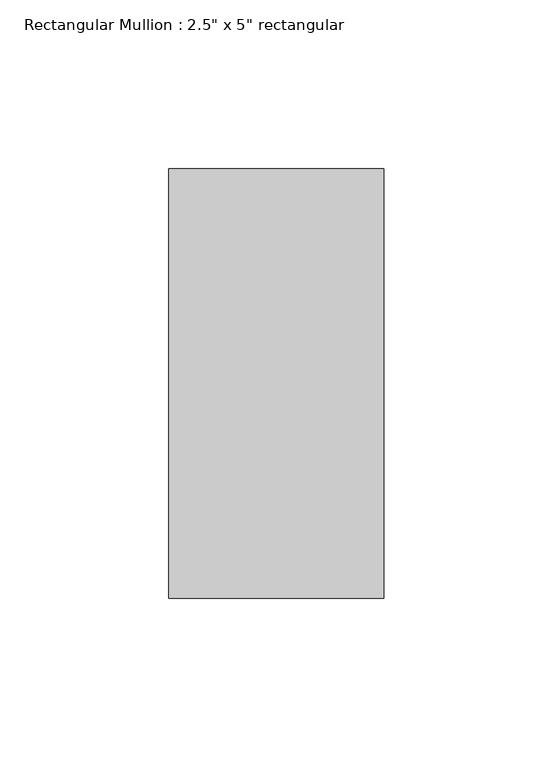
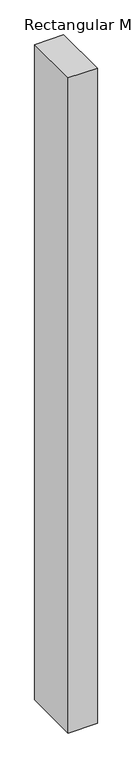
"""IFC4 building model written with IfcOpenShell, lengths in millimetres: member geometry."""

from ifc_helpers import new_model, si_unit, frame, origin, place, context, project, spatial, polyline, outline, extrude, source, transform, mapped, element, save


def member_a31ba1dd(model_context):
    return source(origin(), model_context, "Body", "SweptSolid", [
        extrude(outline(polyline([(0.0, 63.5), (0.0, -63.5), (-63.5, -63.5), (-63.5, 63.5), (0.0, 63.5)])), frame((0.0, 0.0, -1513.786396), z_axis=(0.0, 0.0, 1.0), x_axis=(1.0, 0.0, 0.0)), (0.0, 0.0, 1.0), 1513.786396),
    ])


if __name__ == "__main__":
    model = new_model("IFC4")
    model_context = context("Model", 3, world=origin())
    ifc_project = project(units=[si_unit("LENGTHUNIT", "METRE", prefix="MILLI")], contexts=[model_context])
    site = spatial("IfcSite", under=ifc_project)
    building = spatial("IfcBuilding", under=site)
    placement = place(None, origin())
    member_shape = member_a31ba1dd(model_context)
    element("IfcMember", 1, ObjectType="Rectangular Mullion : 2.5\" x 5\" rectangular", at=placement, inside=building, context=model_context, shape_type="MappedRepresentation", body=[
        mapped(member_shape, transform((0.0, 0.0, 0.0), x_axis=(1.0, 0.0, 0.0), y_axis=(0.0, 1.0, 0.0), z_axis=(0.0, 0.0, 1.0))),
    ])
    save(model, "model.ifc")

# Revit data of these elements
# Type "Rectangular Mullion : 2.5\" x 5\" rectangular"
#   built-in parameter 1007304 = 0.416667 (stored number, unit not read)
#   built-in parameter 1007301 = 0.104167 (stored number, unit not read)
#   built-in parameter 1007300 = 0.104167 (stored number, unit not read)
# Element 1 (IfcMember, "Rectangular Mullion : 2.5\" x 5\" rectangular")
#   Materials on its faces: "Aluminum"
# Materials
#   "Aluminum": class "Metal", colour RGB 247 247 247, transparency 0, Description = "Aluminum 6061", Cost = 0
